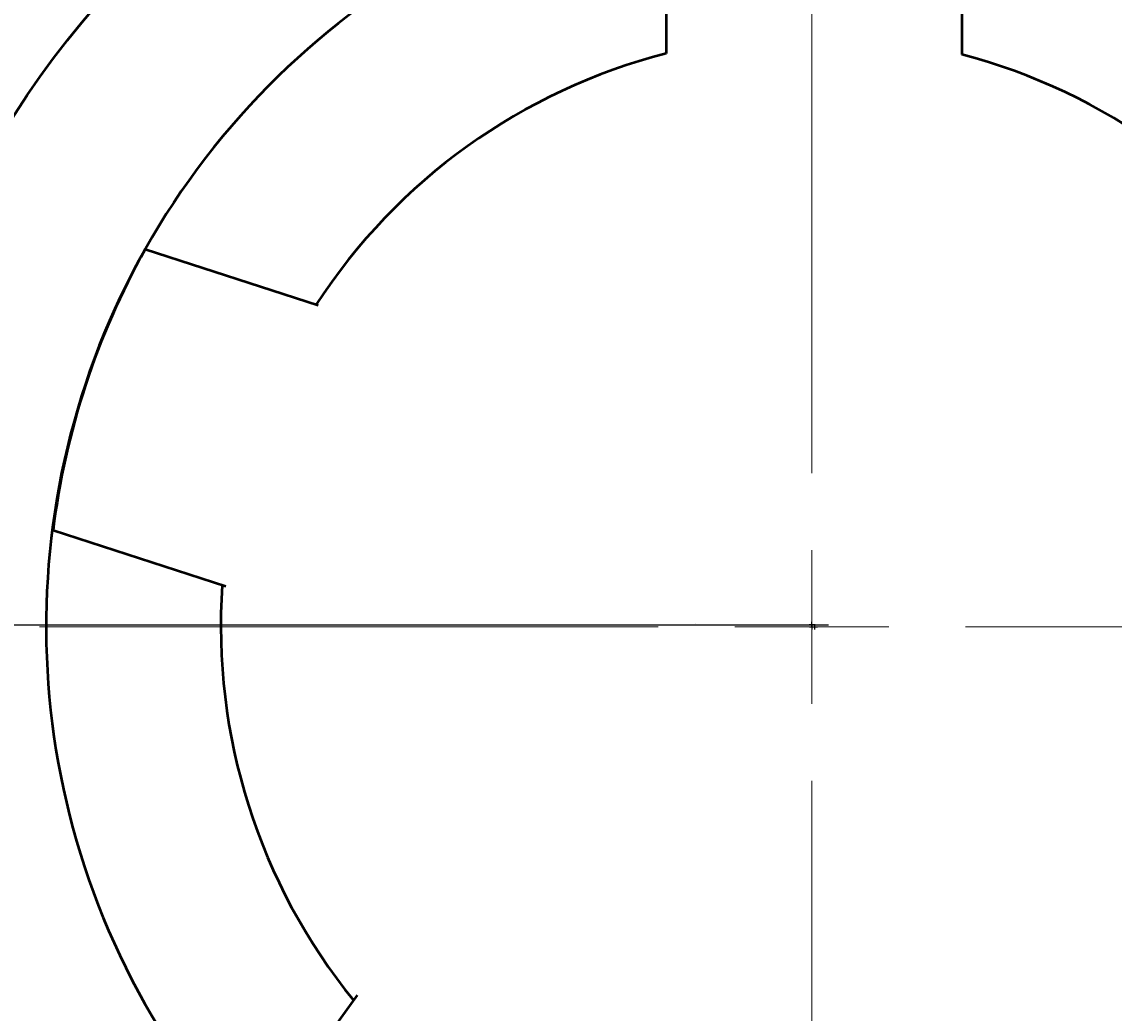
# Model space of a CAD drawing. Units: millimetres. Extents: x -50 to 109, y -46 to 152.
# Tile 3 of 18: x -28 to 9, y -20 to 14. Entities that reach past the tile are written whole.
import ezdxf

# ---------------------------------------------------------------- set-up
doc = ezdxf.new("R2010")
doc.units = ezdxf.units.MM
doc.header["$MEASUREMENT"] = 0
doc.linetypes.add('CENTER', pattern=[50.8, 31.75, -6.35, 6.35, -6.35])
for name, color, linetype, lineweight in [('M-CNTR', 1, 'CENTER', 18), ('M-DIMS', 2, 'Continuous', 25), ('M-OUTL', 7, 'Continuous', 50)]:
    doc.layers.add(name, color=color, linetype=linetype, lineweight=lineweight)
doc.styles.get("Standard").update_dxf_attribs({"font": 'arial.ttf'})
doc.dimstyles.get("Standard").update_dxf_attribs({"dimtxt": 0.18, "dimasz": 0.18, "dimexe": 0.18, "dimexo": 0.0625, "dimgap": 0.09, "dimtad": 0, "dimtih": 1, "dimtoh": 1, "dimdec": 4, "dimzin": 0, "dimdsep": 46, "dimtxsty": 'Standard', "dimcen": 0.09, "dimadec": 0, "dimazin": 0, "dimtfac": 1, "dimtdec": 4, "dimtofl": 0, "dimtmove": 0, "dimatfit": 3, "dimfxl": 1, "dimtolj": 1, "dimtzin": 0, "dimarcsym": 0})

# ---------------------------------------------------------------- blocks, each defined once
blk = doc.blocks.new('*U1')
for p, q in [((-5, 2.851), (-5, -3.294)), ((5, 2.824), (5, -3.323))]:
    blk.add_line(p, q)
blk.add_arc((-0.069, -22.677), 26, 78.7582, 100.9333)
blk = doc.blocks.new('*U2')
at = {"layer": 'M-OUTL', "color": 0, "linetype": 'ByBlock', "lineweight": -2, "transparency": 16777216}
blk.add_blockref('*U1', (-0.855, 15.809), dxfattribs=at)
for p, rotation in [((-22.328, 0.278), 72), ((-14.194, -24.943), 144), ((12.307, -25), 216)]:
    blk.add_blockref('*U1', p, dxfattribs=dict(at, rotation=rotation))
blk = doc.blocks.new('*U6')
at = {"layer": 'M-CNTR', "color": 0, "transparency": 16777216}
for p, q in [((0, 5.2), (0, 36)), ((-26.12, 0), (-5.2, 0)), ((5.2, 0), (26.12, 0)), ((0, -26.12), (0, -5.2))]:
    blk.add_line(p, q, dxfattribs=at)
at = {"layer": 'M-CNTR', "color": 0, "linetype": 'Continuous', "transparency": 16777216}
for p, q in [((0, -2.6), (0, 2.6)), ((-2.6, 0), (2.6, 0))]:
    blk.add_line(p, q, dxfattribs=at)
blk = doc.blocks.new('*D22')
at = {"layer": 'Defpoints', "color": 0, "transparency": 16777216}
for p in [(0.661, 13.074), (-2.483, -26.803)]:
    blk.add_point(p, dxfattribs=at)
at = {"layer": 'M-DIMS', "color": 0, "lineweight": -2, "transparency": 16777216}
for p, q in [((-1.001, -6.864), (-0.821, -6.864)), ((-0.911, -6.954), (-0.911, -6.774)), ((-3.894, -44.69), (-2.498, -26.982)), ((-4.074, -44.69), (-3.894, -44.69))]:
    blk.add_line(p, q, dxfattribs=at)
at = {"layer": 'M-DIMS', "color": 0, "transparency": 16777216}
blk.add_solid([(-2.527, -26.98), (-2.468, -26.984), (-2.483, -26.803)], dxfattribs=at)
at = {"layer": 'M-DIMS', "color": 0, "transparency": 16777216, "insert": (-7.94, -44.69), "char_height": 0.18, "attachment_point": 5}
blk.add_mtext('\\A1;{\\H16.66667x;%%C40}', dxfattribs=at)
blk = doc.blocks.new('*D23')
at = {"layer": 'Defpoints', "color": 0, "transparency": 16777216}
for p in [(24.75, 12.317), (-26.598, -25.885)]:
    blk.add_point(p, dxfattribs=at)
at = {"layer": 'M-DIMS', "color": 0, "lineweight": -2, "transparency": 16777216}
for p, q in [((-1.014, -6.784), (-0.834, -6.784)), ((-0.924, -6.874), (-0.924, -6.694)), ((-30.604, -28.865), (-26.742, -25.992)), ((-30.784, -28.865), (-30.604, -28.865))]:
    blk.add_line(p, q, dxfattribs=at)
at = {"layer": 'M-DIMS', "color": 0, "transparency": 16777216}
blk.add_solid([(-26.76, -25.968), (-26.724, -26.016), (-26.598, -25.885)], dxfattribs=at)
at = {"layer": 'M-DIMS', "color": 0, "transparency": 16777216, "insert": (-34.648, -28.865), "char_height": 0.18, "attachment_point": 5}
blk.add_mtext('\\A1;{\\H16.66667x;%%C64}', dxfattribs=at)
blk = doc.blocks.new('*D24')
at = {"layer": 'Defpoints', "color": 0, "transparency": 16777216}
for p in [(-9.958, 17.477), (8.318, -31.205)]:
    blk.add_point(p, dxfattribs=at)
at = {"layer": 'M-DIMS', "color": 0, "lineweight": -2, "transparency": 16777216}
for p, q in [((-13.793, 27.212), (-13.613, 27.212)), ((-13.613, 27.212), (-10.022, 17.646)), ((-0.91, -6.864), (-0.73, -6.864)), ((-0.82, -6.954), (-0.82, -6.774))]:
    blk.add_line(p, q, dxfattribs=at)
at = {"layer": 'M-DIMS', "color": 0, "transparency": 16777216}
blk.add_solid([(-9.994, 17.656), (-10.05, 17.635), (-9.958, 17.477)], dxfattribs=at)
at = {"layer": 'M-DIMS', "color": 0, "transparency": 16777216, "insert": (-17.649, 27.212), "char_height": 0.18, "attachment_point": 5}
blk.add_mtext('\\A1;{\\H16.66667x;%%C52}', dxfattribs=at)
blk = doc.blocks.new('*D25')
at = {"layer": 'Defpoints', "color": 0, "transparency": 16777216}
for p in [(0.007, 66.376), (-48.373, -6.811), (-0.299, -6.811)]:
    blk.add_point(p, dxfattribs=at)
at = {"layer": 'M-DIMS', "color": 0, "lineweight": -2, "transparency": 16777216}
for p, q in [((-0.056, 66.376), (-48.553, 66.376)), ((-48.373, 66.196), (-48.373, 31.405)), ((-48.373, -6.631), (-48.373, 28.16)), ((-0.361, -6.811), (-48.553, -6.811))]:
    blk.add_line(p, q, dxfattribs=at)
at = {"layer": 'M-DIMS', "color": 0, "transparency": 16777216}
for points in [[(-48.403, 66.196), (-48.343, 66.196), (-48.373, 66.376)], [(-48.403, -6.631), (-48.343, -6.631), (-48.373, -6.811)]]:
    blk.add_solid(points, dxfattribs=at)
at = {"layer": 'M-DIMS', "color": 0, "transparency": 16777216, "insert": (-48.373, 29.782), "char_height": 0.18, "attachment_point": 5}
blk.add_mtext('\\A1;{\\H16.66667x;73}', dxfattribs=at)
blk = doc.blocks.new('*D29')
at = {"layer": 'Defpoints', "color": 0, "transparency": 16777216}
for p in [(21.684, 15.863), (-23.531, -29.431)]:
    blk.add_point(p, dxfattribs=at)
at = {"layer": 'M-DIMS', "color": 0, "lineweight": -2, "transparency": 16777216}
for p, q in [((-1.014, -6.784), (-0.834, -6.784)), ((-0.924, -6.874), (-0.924, -6.694)), ((-37.096, -43.02), (-23.658, -29.559)), ((-37.276, -43.02), (-37.096, -43.02))]:
    blk.add_line(p, q, dxfattribs=at)
at = {"layer": 'M-DIMS', "color": 0, "transparency": 16777216}
blk.add_solid([(-23.68, -29.537), (-23.637, -29.58), (-23.531, -29.431)], dxfattribs=at)
at = {"layer": 'M-DIMS', "color": 0, "transparency": 16777216, "insert": (-37.592, -43.02), "char_height": 0.18, "attachment_point": 5}
blk.add_mtext('\\A1;∅64', dxfattribs=at)

msp = doc.modelspace()

# ---------------------------------------------------------------- linework, layer by layer
at = {"layer": 'M-OUTL'}
msp.add_line((-4.85497, -6.75826), (-4.85497, -6.75888), dxfattribs=at)
msp.add_circle((-0.92366, -6.78396), 32, dxfattribs=at)
for centre, radius, start, end in [((-0.82008, -6.86387), 26, 78.565718, 270.188748), ((-0.91099, -6.86447), 20, 104.311846, 147.003895), ((-0.91099, -6.86447), 20, 32.692944, 75.356698), ((-0.91099, -6.86447), 20, 175.960129, 219.167574)]:
    msp.add_arc(centre, radius, start, end, dxfattribs=at)

# ---------------------------------------------------------------- block references
at = {"layer": 'M-CNTR'}
msp.add_blockref('*U6', (-0.92366, -6.86889), dxfattribs=at)
at = {"layer": 'M-OUTL'}
msp.add_blockref('*U2', (0, 0), dxfattribs=at)

# ---------------------------------------------------------------- dimensions: what is measured, and where the dimension line sits
at = {"layer": 'M-DIMS'}
dim = msp.add_linear_dim(base=(-48.37276, -6.81116), p1=(0.00669, 66.37611), p2=(-0.2986, -6.81116), angle=90, text='{\\H16.66667x;73}', dimstyle='Standard', override={"dimclrd": 0, "dimclre": 0, "dimclrt": 0}, dxfattribs=at)
dim.commit()
dim.dimension.update_dxf_attribs({"geometry": '*D25', "text_midpoint": (-48.37276, 29.78248)})
for p1, p2, text, picture, middle in [((8.31828, -31.20499), (-9.95844, 17.47726), '{\\H16.66667x;%%C52}', '*D24', (-17.64865, 27.21244)), ((0.6614, 13.07362), (-2.48337, -26.80257), '{\\H16.66667x;%%C40}', '*D22', (-7.93965, -44.69043)), ((24.75033, 12.31698), (-26.59765, -25.88491), '{\\H16.66667x;%%C64}', '*D23', (-34.64806, -28.86518))]:
    dim = msp.add_diameter_dim_2p(p1=p1, p2=p2, text=text, dimstyle='Standard', override={"dimclrd": 0, "dimclre": 0, "dimclrt": 0}, dxfattribs=at)
    dim.commit()
    dim.dimension.update_dxf_attribs({"geometry": picture, "text_midpoint": middle, "dimtype": 163})
dim = msp.add_diameter_dim_2p(p1=(21.68387, 15.86332), p2=(-23.53119, -29.43125), dimstyle='Standard', override={"dimdec": 0, "dimlfac": 1, "dimrnd": 0, "dimzin": 0, "dimdsep": 46, "dimlunit": 2}, dxfattribs=at)
dim.commit()
dim.dimension.update_dxf_attribs({"geometry": '*D29', "text_midpoint": (-37.59218, -43.01962), "dimtype": 163})

doc.saveas('drawing.dxf')
